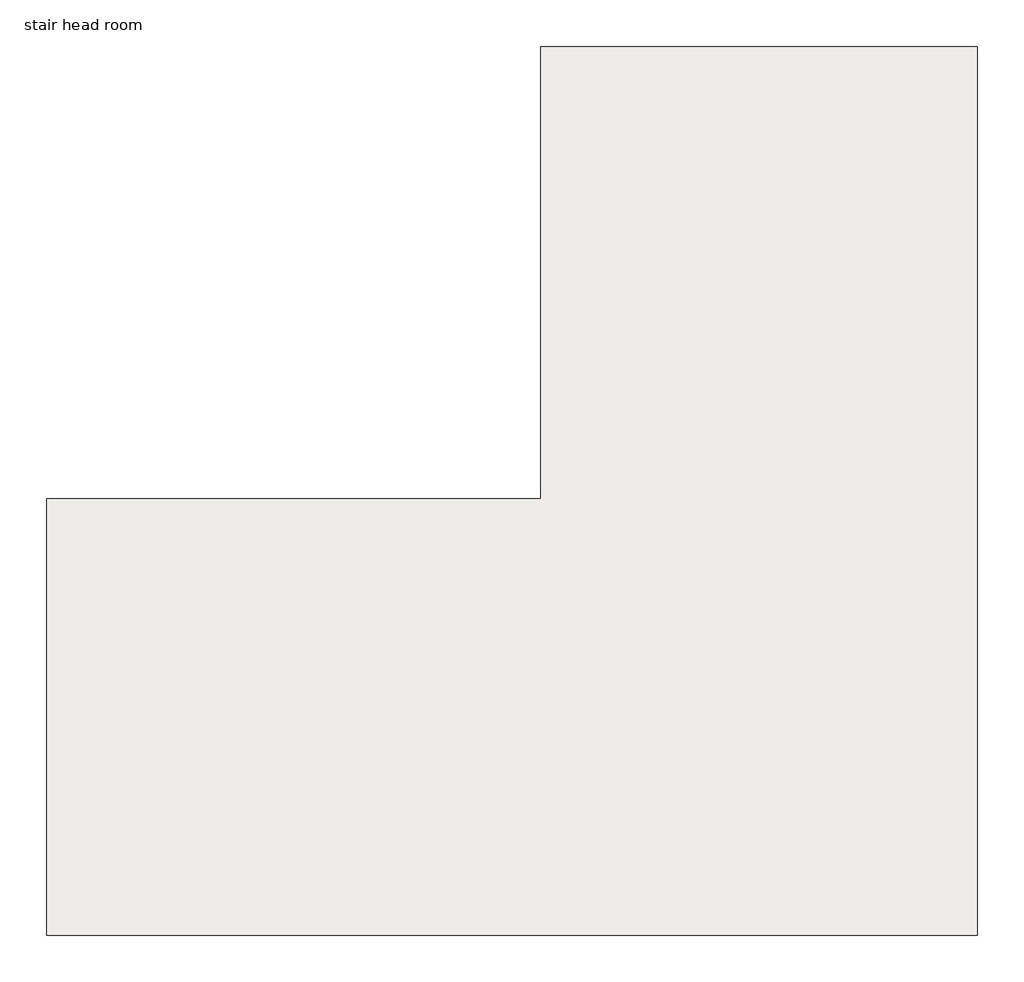
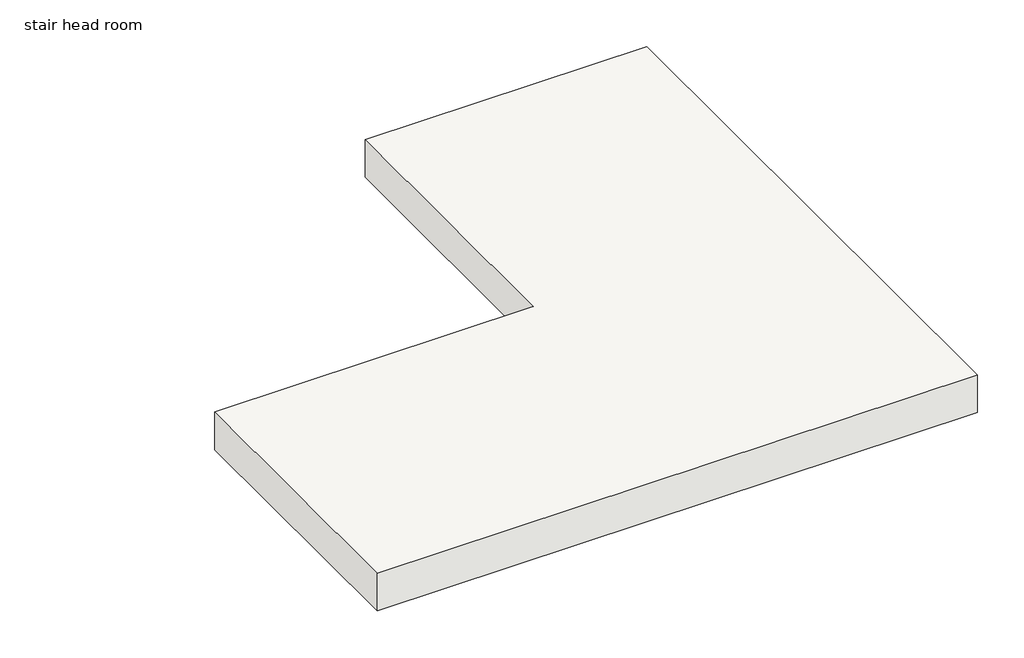
# One storey: 1 slab.
"""IFC4 building model written with IfcOpenShell, lengths in millimetres."""

from ifc_helpers import new_model, si_unit, frame, origin, place, context, project, spatial, polyline, outline, extrude, element, save

model = new_model("IFC4")

# Units and contexts
model_context = context("Model", 3, world=origin())
ifc_project = project(units=[si_unit("LENGTHUNIT", "METRE", prefix="MILLI")], contexts=[model_context])

# Site, building, storey
site = spatial("IfcSite", under=ifc_project)
building = spatial("IfcBuilding", under=site)
storey = spatial("IfcBuildingStorey", under=building, Name="stair head room", Elevation=6553.2)

# Slab
placement = place(None, origin())
element("IfcSlab", 1, ObjectType="Generic - 12\"", at=placement, inside=storey, context=model_context, shape_type="SweptSolid", body=[
    extrude(outline(polyline([(6012.7214491, 8465.3154956), (8456.2808241, 8465.3154956), (8456.2808241, 10700.5154956), (10615.6776991, 10700.5154956), (10615.6776991, 6306.3154956), (6012.7214491, 6306.3154956), (6012.7214491, 8465.3154956)])), frame((0.0, 0.0, 6248.4), z_axis=(0.0, 0.0, 1.0), x_axis=(1.0, 0.0, 0.0)), (0.0, 0.0, 1.0), 304.8),
])

save(model, "model.ifc")

# Revit data of these elements
# Type "Generic - 12\""
#   Assembly Code = "B1010"
#   Function = 0
#   Layers, outside or top first: 1' - 0" no material (function 1)
# Element 1 (IfcSlab, "Generic - 12\"")
#   built-in parameter 1001955 = 1.5708 (stored number, unit not read)
#   Height Offset From Level = 0' - 0"
#   Phase Created = New Construction
#   Materials on its faces: "Default Floor"
# Materials
#   "Default Floor": colour RGB 128 128 128, transparency 0, Cost = 0
